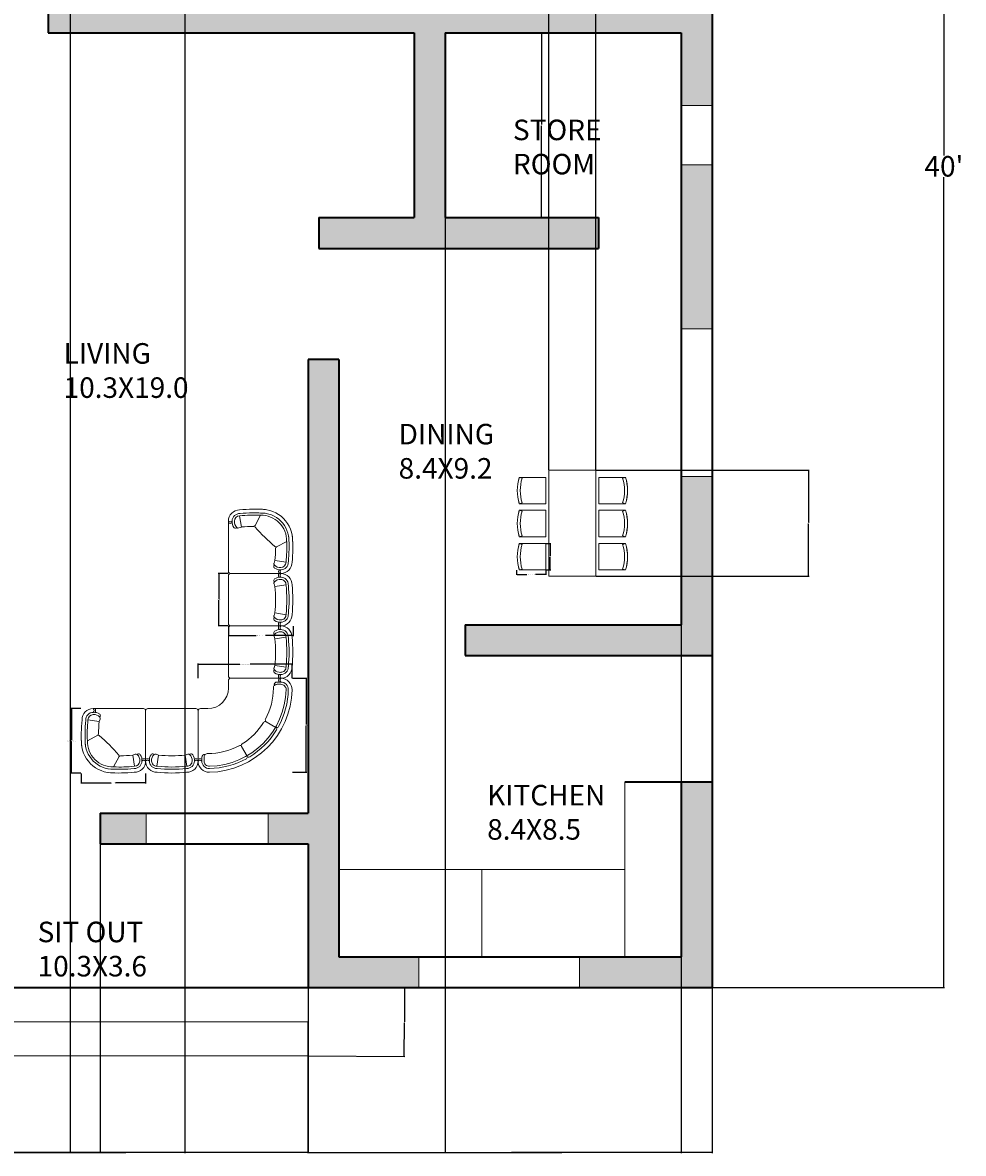
# Model space of a CAD drawing. Units: inches. Extents: x 8 to 486, y -516 to 97.
# Tile 2 of 5: x 211 to 486, y -516 to -185. Entities that reach past the tile are written whole.
import ezdxf

# ---------------------------------------------------------------- set-up
doc = ezdxf.new("R2010")
doc.units = ezdxf.units.IN
doc.header["$MEASUREMENT"] = 0
for name, color, linetype, lineweight in [('A-ANNO-DIMS', 2, 'Continuous', 18), ('A-AREA-IDEN', 7, 'Continuous', 18), ('A-FLOR-CABN', 8, 'Continuous', 18), ('A-FLOR-STRS', 7, 'Continuous', 18), ('A-FURN', 8, 'Continuous', 18), ('A-GLAZ', 4, 'Continuous', 18), ('A-WALL', 7, 'Continuous', 35), ('A-WALL-PATT', 150, 'Continuous', 13)]:
    doc.layers.add(name, color=color, linetype=linetype, lineweight=lineweight)
doc.styles.get("Standard").update_dxf_attribs({"font": 'arial.ttf'})
doc.dimstyles.get("Standard").update_dxf_attribs({"dimtxt": 0.18, "dimasz": 0.18, "dimexe": 0.18, "dimexo": 0.0625, "dimgap": 0.09, "dimtad": 0, "dimtih": 1, "dimtoh": 1, "dimdec": 0, "dimzin": 0, "dimdsep": 46, "dimlunit": 3, "dimtxsty": 'Standard', "dimcen": 0.09, "dimadec": 0, "dimazin": 0, "dimtfac": 1, "dimtdec": 0, "dimtofl": 0, "dimtmove": 0, "dimatfit": 3, "dimfxl": 1, "dimtolj": 1, "dimtzin": 0, "dimarcsym": 0})

# ---------------------------------------------------------------- blocks, each defined once
blk = doc.blocks.new('*D2')
at = {"layer": 'A-ANNO-DIMS', "color": 0, "lineweight": -2, "transparency": 16777216}
for p, q in [((412.19, 12.74), (480.06, 12.74)), ((479.88, 12.56), (479.88, -224.11)), ((479.88, -467.08), (479.88, -230.42)), ((412.19, -467.26), (480.06, -467.26))]:
    blk.add_line(p, q, dxfattribs=at)
at = {"layer": 'A-ANNO-DIMS', "color": 0, "transparency": 16777216}
for points in [[(479.85, 12.56), (479.91, 12.56), (479.88, 12.74)], [(479.85, -467.08), (479.91, -467.08), (479.88, -467.26)]]:
    blk.add_solid(points, dxfattribs=at)
at = {"layer": 'Defpoints', "color": 0, "transparency": 16777216}
for p in [(412.13, 12.74), (412.13, -467.26), (479.88, -467.26)]:
    blk.add_point(p, dxfattribs=at)
at = {"layer": 'A-ANNO-DIMS', "color": 0, "transparency": 16777216, "insert": (479.88, -227.26), "char_height": 6, "attachment_point": 5}
blk.add_mtext("\\A1;40'", dxfattribs=at)
blk = doc.blocks.new('A$C707258B2')
at = {"color": 0}
for p, q in [((0.404, 0.342), (1.074, 0.342)), ((1.104, 0.312), (1.104, 0.212)), ((0.404, 0.292), (0.454, 0.292)), ((0.404, 0.262), (0.454, 0.262)), ((1.479, -0.063), (1.379, -0.063)), ((1.509, -0.763), (1.509, -0.093)), ((0.6, -0.238), (0.47, -0.313)), ((0.929, -0.567), (0.854, -0.697)), ((1.429, -0.763), (1.429, -0.713)), ((1.459, -0.763), (1.459, -0.712))]:
    blk.add_line(p, q, dxfattribs=at)
for centre, radius, start, end in [((0.404, 0.192), 0.15, 90, 181.1754), ((0.378, 0.317), 0.0362, 316.3972, 43.6028), ((0.368, 0.317), 0.0662, 337.8298, 22.1702), ((1.074, 0.312), 0.03, 360, 90), ((1.379, 0.212), 1.125, 181.1754, 268.8246), ((0.404, 0.192), 0.1, 90, 181.1754), ((1.379, 0.212), 1.075, 181.1754, 208.6357), ((0.404, 0.192), 0.07, 90, 181.1754), ((1.379, 0.212), 1.045, 181.1754, 268.8246), ((0.455, 0.256), 0.0357, 345.4262, 90.5555), ((0.454, 0.212), 0.05, 360, 90), ((1.379, 0.212), 0.875, 180, 208.4082), ((1.379, 0.212), 0.275, 180, 270), ((1.479, -0.093), 0.03, 360, 90), ((0.587, -0.216), 0.025, 300, 28.4082), ((0.612, -0.259), 0.025, 31.5918, 120), ((1.379, 0.212), 0.875, 211.5918, 238.4082), ((0.457, -0.291), 0.025, 208.6357, 300), ((0.482, -0.334), 0.025, 120, 211.3643), ((1.379, 0.212), 1.075, 211.3643, 238.6357), ((0.907, -0.555), 0.025, 330, 58.4082), ((0.951, -0.58), 0.025, 61.5918, 150), ((1.379, 0.212), 0.875, 241.5918, 270), ((0.832, -0.685), 0.025, 238.6357, 330), ((0.876, -0.71), 0.025, 150, 241.3643), ((1.379, 0.212), 1.075, 241.3643, 268.8246), ((1.379, -0.713), 0.05, 360, 90), ((1.425, -0.709), 0.0336, 354.6301, 109.3883), ((1.484, -0.799), 0.0662, 67.8298, 112.1702), ((1.484, -0.789), 0.0362, 46.3972, 133.6028), ((1.359, -0.763), 0.15, 268.8246, 360), ((1.359, -0.763), 0.1, 268.8246, 360), ((1.359, -0.763), 0.07, 268.8246, 360)]:
    blk.add_arc(centre, radius, start, end, dxfattribs=at)
blk = doc.blocks.new('part 01')
at = {"color": 0}
for p, q in [((-670, 700), (0, 700)), ((30, 30), (30, 670)), ((-591, 527), (-740, 550)), ((-591, 527), (-579, 561)), ((-591, 173), (-740, 150)), ((-591, 173), (-579, 139)), ((-670, 0), (0, 0))]:
    blk.add_line(p, q, dxfattribs=at)
for centre, radius, start, end in [((-670, 550), 150, 90, 181.1754), ((-670, 550), 100, 90, 181.1754), ((-670, 550), 70, 90, 181.1754), ((-660, 518), 133, 56.0897, 95.6132), ((-696, 675), 36.2, 316.3972, 43.6028), ((-660, 518), 103, 42.0066, 95.6132), ((-706, 675), 66.2, 337.8298, 22.1702), ((-600, 607), 25, 332.9608, 56.0897), ((0, 670), 30, 0, 90), ((1178, 350), 2008, 174.2835, 185.7165), ((1178, 350), 1958, 174.2835, 185.7165), ((1178, 350), 1928, 174.2835, 185.7165), ((1178, 350), 1778, 174.2835, 185.7165), ((-625, 620), 53.2, 321.0017, 332.9608), ((-602, 570), 25, 340, 42.0066), ((-670, 150), 150, 178.8246, 270), ((-670, 150), 100, 178.8246, 270), ((-670, 150), 70, 178.8246, 270), ((-660, 182), 133, 264.3868, 303.9103), ((-660, 182), 103, 264.3868, 317.9934), ((-696, 25), 36.2, 316.3972, 43.6028), ((-706, 25), 66.2, 337.8298, 22.1702), ((-600, 93), 25, 303.9103, 27.0392), ((-602, 130), 25, 317.9934, 20), ((-625, 80), 53.2, 27.0392, 38.9983), ((0, 30), 30, 270, 0)]:
    blk.add_arc(centre, radius, start, end, dxfattribs=at)
blk = doc.blocks.new('part02')
at = {"color": 0}
for p, q in [((0, -670), (0, 0)), ((30, 30), (700, 30)), ((621, -143), (609, -109)), ((621, -143), (770, -120)), ((640, -326), (778, -399)), ((173, -591), (139, -579)), ((173, -591), (150, -740)), ((356, -610), (429, -748))]:
    blk.add_line(p, q, dxfattribs=at)
for centre, radius, start, end in [((30, 0), 30, 90, 180), ((726, 5), 56.2, 153.6122, 206.6666), ((726, 5), 36.2, 136.3972, 223.6028), ((700, -120), 150, 0, 90), ((630, -63), 25, 123.9103, 207.0392), ((655, -50), 53.2, 207.0392, 218.9983), ((632, -100), 25, 137.9934, 200), ((690, -152), 103, 84.3868, 137.9934), ((689, -151), 132, 85.4378, 123.9887), ((-1148, -320), 1778, 0.3836, 5.7165), ((700, -121), 101, 357.5006, 89.858), ((700, -120), 70, 0, 90), ((-1228, -320), 2008, 357.7349, 5.7032), ((-1148, -320), 1958, 355.8657, 5.7165), ((-1148, -320), 2008, 355.818, 5.7165), ((2220, -2190), 2454, 130.6961, 139.3039), ((439, -409), 419, 268.2181, 1.7819), ((439, -409), 369, 268.2181, 1.7819), ((439, -409), 339, 268.2181, 1.7819), ((632, -344), 20, 62, 130.6961), ((650, -308), 20, 180.3836, 242), ((182, -660), 133, 146.0897, 185.6132), ((93, -600), 25, 62.9608, 146.0897), ((182, -660), 103, 132.0066, 185.6132), ((80, -625), 53.2, 51.0017, 62.9608), ((130, -602), 25, 70, 132.0066), ((350, 1178), 1778, 264.2835, 269.6164), ((338, -620), 20, 28, 89.6164), ((374, -602), 20, 139.3039, 208), ((25, -696), 56.2, 63.3334, 116.3878), ((25, -696), 36.2, 46.3972, 133.6028), ((150, -670), 150, 180, 271.1754), ((150, -670), 100, 180, 271.1754), ((150, -670), 70, 180, 270), ((350, 1258), 2008, 264.2968, 272.2651), ((350, 1178), 2008, 264.2835, 274.182), ((350, 1178), 1958, 264.2835, 274.1343)]:
    blk.add_arc(centre, radius, start, end, dxfattribs=at)
blk = doc.blocks.new('CHAIR-DINING')
for p, q in [((0.6, 7.75), (1.42, 7.49)), ((0.6, 0), (1.42, 0.26))]:
    blk.add_line(p, q)
blk.add_lwpolyline([(0.6, 7.75), (8.35, 7.75), (8.35, 0), (0.6, 0, -0.153703), (0.6, 7.75)], format="xyb")
for radius in [12.78, 11.92]:
    blk.add_arc((12.79, 3.88), radius, 162.3544, 197.6456)
blk = doc.blocks.new('*D13')
at = {"layer": 'A-ANNO-DIMS', "color": 0, "lineweight": -2, "transparency": 16777216}
for p, q in [((355.03, -345.29), (355.03, -346.69)), ((355.21, -346.51), (358.03, -346.51)), ((363.4, -346.51), (360.58, -346.51)), ((363.58, -345.29), (363.58, -346.69))]:
    blk.add_line(p, q, dxfattribs=at)
at = {"layer": 'A-ANNO-DIMS', "color": 0, "transparency": 16777216}
for points in [[(355.21, -346.48), (355.21, -346.54), (355.03, -346.51)], [(363.4, -346.48), (363.4, -346.54), (363.58, -346.51)]]:
    blk.add_solid(points, dxfattribs=at)
at = {"layer": 'Defpoints', "color": 0, "transparency": 16777216}
for p in [(355.03, -345.23), (363.58, -345.23), (363.58, -346.51)]:
    blk.add_point(p, dxfattribs=at)
at = {"layer": 'A-ANNO-DIMS', "color": 0, "transparency": 16777216, "insert": (359.3, -346.51), "char_height": 0.18, "attachment_point": 5}
blk.add_mtext('\\A1;CHAIR 0\'-8 1/2" TYP.', dxfattribs=at)
blk = doc.blocks.new('*D14')
at = {"layer": 'A-ANNO-DIMS', "color": 0, "lineweight": -2, "transparency": 16777216}
for p, q in [((363.64, -337.48), (365.04, -337.48)), ((364.86, -337.66), (364.86, -341.17)), ((364.86, -345.05), (364.86, -341.53)), ((363.64, -345.23), (365.04, -345.23))]:
    blk.add_line(p, q, dxfattribs=at)
at = {"layer": 'A-ANNO-DIMS', "color": 0, "transparency": 16777216}
for points in [[(364.83, -337.66), (364.89, -337.66), (364.86, -337.48)], [(364.83, -345.05), (364.89, -345.05), (364.86, -345.23)]]:
    blk.add_solid(points, dxfattribs=at)
at = {"layer": 'Defpoints', "color": 0, "transparency": 16777216}
for p in [(363.58, -337.48), (364.86, -337.48), (363.58, -345.23)]:
    blk.add_point(p, dxfattribs=at)
at = {"layer": 'A-ANNO-DIMS', "color": 0, "transparency": 16777216, "insert": (364.86, -341.35), "char_height": 0.18, "attachment_point": 5}
blk.add_mtext('\\A1;0\'-8" TYP.', dxfattribs=at)
blk = doc.blocks.new('*D15')
at = {"layer": 'A-ANNO-DIMS', "color": 0, "lineweight": -2, "transparency": 16777216}
for p, q in [((270.85, -361.64), (270.85, -364.59)), ((289.73, -361.64), (289.73, -364.59)), ((271.03, -364.41), (278.91, -364.41)), ((289.55, -364.41), (281.67, -364.41))]:
    blk.add_line(p, q, dxfattribs=at)
at = {"layer": 'A-ANNO-DIMS', "color": 0, "transparency": 16777216}
for points in [[(271.03, -364.38), (271.03, -364.44), (270.85, -364.41)], [(289.55, -364.38), (289.55, -364.44), (289.73, -364.41)]]:
    blk.add_solid(points, dxfattribs=at)
at = {"layer": 'Defpoints', "color": 0, "transparency": 16777216}
for p in [(270.85, -361.58), (289.73, -361.58), (270.85, -364.41)]:
    blk.add_point(p, dxfattribs=at)
at = {"layer": 'A-ANNO-DIMS', "color": 0, "transparency": 16777216, "insert": (280.29, -364.41), "char_height": 0.18, "attachment_point": 5}
blk.add_mtext('\\A1;SOFA SEAT 1\'-7" TYP.', dxfattribs=at)
blk = doc.blocks.new('*D16')
at = {"layer": 'A-ANNO-DIMS', "color": 0, "lineweight": -2, "transparency": 16777216}
for p, q in [((270.78, -346.26), (267.83, -346.26)), ((268.01, -346.44), (268.01, -353.74)), ((268.01, -361.4), (268.01, -354.1)), ((270.78, -361.58), (267.83, -361.58))]:
    blk.add_line(p, q, dxfattribs=at)
at = {"layer": 'A-ANNO-DIMS', "color": 0, "transparency": 16777216}
for points in [[(267.98, -346.44), (268.04, -346.44), (268.01, -346.26)], [(267.98, -361.4), (268.04, -361.4), (268.01, -361.58)]]:
    blk.add_solid(points, dxfattribs=at)
at = {"layer": 'Defpoints', "color": 0, "transparency": 16777216}
for p in [(268.01, -346.26), (270.85, -346.26), (270.85, -361.58)]:
    blk.add_point(p, dxfattribs=at)
at = {"layer": 'A-ANNO-DIMS', "color": 0, "transparency": 16777216, "insert": (268.01, -353.92), "char_height": 0.18, "attachment_point": 5}
blk.add_mtext('\\A1;1\'-3 1/2" TYP.', dxfattribs=at)
blk = doc.blocks.new('*D17')
at = {"layer": 'A-ANNO-DIMS', "color": 0, "lineweight": -2, "transparency": 16777216}
for p, q in [((227.73, -385.75), (224.78, -385.75)), ((224.96, -385.93), (224.96, -395.01)), ((224.96, -404.45), (224.96, -395.38)), ((227.73, -404.63), (224.78, -404.63))]:
    blk.add_line(p, q, dxfattribs=at)
at = {"layer": 'A-ANNO-DIMS', "color": 0, "transparency": 16777216}
for points in [[(224.93, -385.93), (224.99, -385.93), (224.96, -385.75)], [(224.93, -404.45), (224.99, -404.45), (224.96, -404.63)]]:
    blk.add_solid(points, dxfattribs=at)
at = {"layer": 'Defpoints', "color": 0, "transparency": 16777216}
for p in [(224.96, -385.75), (227.79, -385.75), (227.79, -404.63)]:
    blk.add_point(p, dxfattribs=at)
at = {"layer": 'A-ANNO-DIMS', "color": 0, "transparency": 16777216, "insert": (224.96, -395.19), "char_height": 0.18, "attachment_point": 5}
blk.add_mtext('\\A1;SOFA END 1\'-7" TYP.', dxfattribs=at)
blk = doc.blocks.new('*D18')
at = {"layer": 'A-ANNO-DIMS', "color": 0, "lineweight": -2, "transparency": 16777216}
for p, q in [((227.79, -404.69), (227.79, -407.64)), ((246.67, -404.69), (246.67, -407.64)), ((227.97, -407.46), (236.6, -407.46)), ((246.49, -407.46), (237.86, -407.46))]:
    blk.add_line(p, q, dxfattribs=at)
at = {"layer": 'A-ANNO-DIMS', "color": 0, "transparency": 16777216}
for points in [[(227.97, -407.43), (227.97, -407.49), (227.79, -407.46)], [(246.49, -407.43), (246.49, -407.49), (246.67, -407.46)]]:
    blk.add_solid(points, dxfattribs=at)
at = {"layer": 'Defpoints', "color": 0, "transparency": 16777216}
for p in [(227.79, -404.63), (246.67, -404.63), (227.79, -407.46)]:
    blk.add_point(p, dxfattribs=at)
at = {"layer": 'A-ANNO-DIMS', "color": 0, "transparency": 16777216, "insert": (237.23, -407.46), "char_height": 0.18, "attachment_point": 5}
blk.add_mtext('\\A1;1\'-7" TYP.', dxfattribs=at)
blk = doc.blocks.new('*D19')
at = {"layer": 'A-ANNO-DIMS', "color": 0, "lineweight": -2, "transparency": 16777216}
for p, q in [((261.99, -376.83), (261.99, -372.59)), ((262.17, -372.77), (274.23, -372.77)), ((289.28, -372.77), (277.22, -372.77)), ((289.46, -376.83), (289.46, -372.59))]:
    blk.add_line(p, q, dxfattribs=at)
at = {"layer": 'A-ANNO-DIMS', "color": 0, "transparency": 16777216}
for points in [[(262.17, -372.74), (262.17, -372.8), (261.99, -372.77)], [(289.28, -372.74), (289.28, -372.8), (289.46, -372.77)]]:
    blk.add_solid(points, dxfattribs=at)
at = {"layer": 'Defpoints', "color": 0, "transparency": 16777216}
for p in [(261.99, -372.77), (261.99, -376.89), (289.46, -376.89)]:
    blk.add_point(p, dxfattribs=at)
at = {"layer": 'A-ANNO-DIMS', "color": 0, "transparency": 16777216, "insert": (275.72, -372.77), "char_height": 0.18, "attachment_point": 5}
blk.add_mtext('\\A1;SOFA CORNER 2\'-3 1/2"', dxfattribs=at)
blk = doc.blocks.new('*D20')
at = {"layer": 'A-ANNO-DIMS', "color": 0, "lineweight": -2, "transparency": 16777216}
for p, q in [((289.52, -376.89), (293.76, -376.89)), ((293.58, -377.07), (293.58, -390.44)), ((293.58, -404.18), (293.58, -390.81)), ((289.52, -404.36), (293.76, -404.36))]:
    blk.add_line(p, q, dxfattribs=at)
at = {"layer": 'A-ANNO-DIMS', "color": 0, "transparency": 16777216}
for points in [[(293.55, -377.07), (293.61, -377.07), (293.58, -376.89)], [(293.55, -404.18), (293.61, -404.18), (293.58, -404.36)]]:
    blk.add_solid(points, dxfattribs=at)
at = {"layer": 'Defpoints', "color": 0, "transparency": 16777216}
for p in [(289.46, -376.89), (293.58, -376.89), (289.46, -404.36)]:
    blk.add_point(p, dxfattribs=at)
at = {"layer": 'A-ANNO-DIMS', "color": 0, "transparency": 16777216, "insert": (293.58, -390.63), "char_height": 0.18, "attachment_point": 5}
blk.add_mtext('\\A1;2\'-3 1/2"', dxfattribs=at)
blk = doc.blocks.new('*D22')
at = {"layer": 'A-ANNO-DIMS', "color": 0, "lineweight": -2, "transparency": 16777216}
for p, q in [((162.13, -487.33), (162.13, -515.64)), ((294.01, -487.33), (294.01, -515.64)), ((162.31, -515.46), (227.68, -515.46)), ((293.83, -515.46), (228.46, -515.46))]:
    blk.add_line(p, q, dxfattribs=at)
at = {"layer": 'A-ANNO-DIMS', "color": 0, "transparency": 16777216}
for points in [[(162.31, -515.43), (162.31, -515.49), (162.13, -515.46)], [(293.83, -515.43), (293.83, -515.49), (294.01, -515.46)]]:
    blk.add_solid(points, dxfattribs=at)
at = {"layer": 'Defpoints', "color": 0, "transparency": 16777216}
for p in [(162.13, -487.26), (294.01, -487.26), (294.01, -515.46)]:
    blk.add_point(p, dxfattribs=at)
at = {"layer": 'A-ANNO-DIMS', "color": 0, "transparency": 16777216, "insert": (228.07, -515.46), "char_height": 0.18, "attachment_point": 5}
blk.add_mtext('\\A1;11\'-0"', dxfattribs=at)
blk = doc.blocks.new('*D23')
at = {"layer": 'A-ANNO-DIMS', "color": 0, "lineweight": -2, "transparency": 16777216}
for p, q in [((294.13, -467.33), (294.13, -515.64)), ((412.13, -467.33), (412.13, -515.64)), ((294.31, -515.46), (352.73, -515.46)), ((411.95, -515.46), (353.53, -515.46))]:
    blk.add_line(p, q, dxfattribs=at)
at = {"layer": 'A-ANNO-DIMS', "color": 0, "transparency": 16777216}
for points in [[(294.31, -515.43), (294.31, -515.49), (294.13, -515.46)], [(411.95, -515.43), (411.95, -515.49), (412.13, -515.46)]]:
    blk.add_solid(points, dxfattribs=at)
at = {"layer": 'Defpoints', "color": 0, "transparency": 16777216}
for p in [(294.13, -467.26), (412.13, -467.26), (412.13, -515.46)]:
    blk.add_point(p, dxfattribs=at)
at = {"layer": 'A-ANNO-DIMS', "color": 0, "transparency": 16777216, "insert": (353.13, -515.46), "char_height": 0.18, "attachment_point": 5}
blk.add_mtext('\\A1;9\'-10"', dxfattribs=at)
blk = doc.blocks.new('*D25')
at = {"layer": 'A-ANNO-DIMS', "color": 0, "lineweight": -2, "transparency": 16777216}
for p, q in [((294.19, -467.27), (322.51, -467.42)), ((322.33, -467.6), (322.27, -477.24)), ((322.21, -487.24), (322.27, -477.61)), ((294.08, -487.27), (322.39, -487.42))]:
    blk.add_line(p, q, dxfattribs=at)
at = {"layer": 'A-ANNO-DIMS', "color": 0, "transparency": 16777216}
for points in [[(322.3, -467.6), (322.36, -467.6), (322.33, -467.42)], [(322.18, -487.24), (322.24, -487.24), (322.21, -487.42)]]:
    blk.add_solid(points, dxfattribs=at)
at = {"layer": 'Defpoints', "color": 0, "transparency": 16777216}
for p in [(294.13, -467.26), (294.01, -487.26), (322.21, -487.42)]:
    blk.add_point(p, dxfattribs=at)
at = {"layer": 'A-ANNO-DIMS', "color": 0, "transparency": 16777216, "insert": (322.27, -477.42), "char_height": 0.18, "attachment_point": 5}
blk.add_mtext('\\A1;1\'-8"', dxfattribs=at)
blk = doc.blocks.new('*D30')
at = {"layer": 'A-ANNO-DIMS', "color": 0, "lineweight": -2, "transparency": 16777216}
for p, q in [((224.63, -103.93), (224.63, -515.64)), ((258.13, -103.93), (258.13, -515.64)), ((224.81, -515.46), (240.84, -515.46)), ((257.95, -515.46), (241.92, -515.46))]:
    blk.add_line(p, q, dxfattribs=at)
at = {"layer": 'A-ANNO-DIMS', "color": 0, "transparency": 16777216}
for points in [[(224.81, -515.43), (224.81, -515.49), (224.63, -515.46)], [(257.95, -515.43), (257.95, -515.49), (258.13, -515.46)]]:
    blk.add_solid(points, dxfattribs=at)
at = {"layer": 'Defpoints', "color": 0, "transparency": 16777216}
for p in [(224.63, -103.87), (258.13, -103.87), (258.13, -515.46)]:
    blk.add_point(p, dxfattribs=at)
at = {"layer": 'A-ANNO-DIMS', "color": 0, "transparency": 16777216, "insert": (241.38, -515.46), "char_height": 0.18, "attachment_point": 5}
blk.add_mtext('\\A1;2\'-9 1/2"', dxfattribs=at)
blk = doc.blocks.new('*D32')
at = {"layer": 'A-ANNO-DIMS', "color": 0, "lineweight": -2, "transparency": 16777216}
for p, q in [((334.13, -188.33), (334.13, -515.64)), ((403.13, -188.33), (403.13, -515.64)), ((334.31, -515.46), (368.3, -515.46)), ((402.95, -515.46), (368.96, -515.46))]:
    blk.add_line(p, q, dxfattribs=at)
at = {"layer": 'A-ANNO-DIMS', "color": 0, "transparency": 16777216}
for points in [[(334.31, -515.43), (334.31, -515.49), (334.13, -515.46)], [(402.95, -515.43), (402.95, -515.49), (403.13, -515.46)]]:
    blk.add_solid(points, dxfattribs=at)
at = {"layer": 'Defpoints', "color": 0, "transparency": 16777216}
for p in [(334.13, -188.26), (403.13, -188.26), (403.13, -515.46)]:
    blk.add_point(p, dxfattribs=at)
at = {"layer": 'A-ANNO-DIMS', "color": 0, "transparency": 16777216, "insert": (368.63, -515.46), "char_height": 0.18, "attachment_point": 5}
blk.add_mtext('\\A1;5\'-9"', dxfattribs=at)
blk = doc.blocks.new('*D33')
at = {"layer": 'A-ANNO-DIMS', "color": 0, "lineweight": -2, "transparency": 16777216}
for p, q in [((334.19, -188.26), (362.51, -188.26)), ((362.33, -188.44), (362.33, -215.08)), ((362.33, -242.08), (362.33, -215.45)), ((334.19, -242.26), (362.51, -242.26))]:
    blk.add_line(p, q, dxfattribs=at)
at = {"layer": 'A-ANNO-DIMS', "color": 0, "transparency": 16777216}
for points in [[(362.3, -188.44), (362.36, -188.44), (362.33, -188.26)], [(362.3, -242.08), (362.36, -242.08), (362.33, -242.26)]]:
    blk.add_solid(points, dxfattribs=at)
at = {"layer": 'Defpoints', "color": 0, "transparency": 16777216}
for p in [(334.13, -188.26), (334.13, -242.26), (362.33, -242.26)]:
    blk.add_point(p, dxfattribs=at)
at = {"layer": 'A-ANNO-DIMS', "color": 0, "transparency": 16777216, "insert": (362.33, -215.26), "char_height": 0.18, "attachment_point": 5}
blk.add_mtext('\\A1;4\'-6"', dxfattribs=at)
blk = doc.blocks.new('*D34')
at = {"layer": 'A-ANNO-DIMS', "color": 0, "lineweight": -2, "transparency": 16777216}
for p, q in [((171.13, -425.33), (171.13, -515.64)), ((233.38, -425.33), (233.38, -515.64)), ((171.31, -515.46), (201.92, -515.46)), ((233.2, -515.46), (202.58, -515.46))]:
    blk.add_line(p, q, dxfattribs=at)
at = {"layer": 'A-ANNO-DIMS', "color": 0, "transparency": 16777216}
for points in [[(171.31, -515.43), (171.31, -515.49), (171.13, -515.46)], [(233.2, -515.43), (233.2, -515.49), (233.38, -515.46)]]:
    blk.add_solid(points, dxfattribs=at)
at = {"layer": 'Defpoints', "color": 0, "transparency": 16777216}
for p in [(171.13, -425.26), (233.38, -425.26), (233.38, -515.46)]:
    blk.add_point(p, dxfattribs=at)
at = {"layer": 'A-ANNO-DIMS', "color": 0, "transparency": 16777216, "insert": (202.25, -515.46), "char_height": 0.18, "attachment_point": 5}
blk.add_mtext('\\A1;5\'-2"', dxfattribs=at)
blk = doc.blocks.new('*D36')
at = {"layer": 'A-ANNO-DIMS', "color": 0, "lineweight": -2, "transparency": 16777216}
for p, q in [((364.45, -315.96), (364.45, 41.12)), ((364.63, 40.94), (371.02, 40.94)), ((378.05, 40.94), (371.66, 40.94)), ((378.23, -315.96), (378.23, 41.12))]:
    blk.add_line(p, q, dxfattribs=at)
at = {"layer": 'A-ANNO-DIMS', "color": 0, "transparency": 16777216}
for points in [[(364.63, 40.97), (364.63, 40.91), (364.45, 40.94)], [(378.05, 40.97), (378.05, 40.91), (378.23, 40.94)]]:
    blk.add_solid(points, dxfattribs=at)
at = {"layer": 'Defpoints', "color": 0, "transparency": 16777216}
for p in [(378.23, 40.94), (364.45, -316.02), (378.23, -316.02)]:
    blk.add_point(p, dxfattribs=at)
at = {"layer": 'A-ANNO-DIMS', "color": 0, "transparency": 16777216, "insert": (371.34, 40.94), "char_height": 0.18, "attachment_point": 5}
blk.add_mtext('\\A1;1\'-2"', dxfattribs=at)
blk = doc.blocks.new('*D37')
at = {"layer": 'A-ANNO-DIMS', "color": 0, "lineweight": -2, "transparency": 16777216}
for p, q in [((378.29, -316.02), (440.51, -316.02)), ((440.33, -316.2), (440.33, -331.34)), ((440.33, -346.84), (440.33, -331.7)), ((378.29, -347.02), (440.51, -347.02))]:
    blk.add_line(p, q, dxfattribs=at)
at = {"layer": 'A-ANNO-DIMS', "color": 0, "transparency": 16777216}
for points in [[(440.3, -316.2), (440.36, -316.2), (440.33, -316.02)], [(440.3, -346.84), (440.36, -346.84), (440.33, -347.02)]]:
    blk.add_solid(points, dxfattribs=at)
at = {"layer": 'Defpoints', "color": 0, "transparency": 16777216}
for p in [(378.23, -316.02), (378.23, -347.02), (440.33, -347.02)]:
    blk.add_point(p, dxfattribs=at)
at = {"layer": 'A-ANNO-DIMS', "color": 0, "transparency": 16777216, "insert": (440.33, -331.52), "char_height": 0.18, "attachment_point": 5}
blk.add_mtext('\\A1;2\'-7"', dxfattribs=at)

msp = doc.modelspace()

# ---------------------------------------------------------------- hatches: boundary and pattern name
at = {"layer": 'A-WALL-PATT'}
h = msp.add_hatch(color=256, dxfattribs=at)
h.dxf.hatch_style = 1
h.paths.add_polyline_path([(91.21, 12.74), (37.13, 12.74), (37.13, -29.65), (46.13, -29.65), (46.13, 3.74), (91.21, 3.74)])
h.paths.add_polyline_path([(211.13, 12.74), (137.85, 12.74), (137.85, 3.74), (182.13, 3.74), (182.13, -73.87), (191.13, -73.87), (191.13, 3.74), (211.13, 3.74)])
h.paths.add_polyline_path([(306.98, 12.74), (234.7, 12.74), (234.7, 3.74), (306.98, 3.74)])
h.paths.add_polyline_path([(267.13, 3.74), (258.13, 3.74), (258.13, -129.26), (267.13, -129.26)])
h.paths.add_polyline_path([(412.13, 12.74), (361.49, 12.74), (361.49, 3.74), (403.13, 3.74), (403.13, -35.28), (412.13, -35.28)])
h.paths.add_polyline_path([(379.01, -120.26), (297.29, -120.26), (297.29, -129.26), (325.13, -129.26), (325.13, -179.26), (218.14, -179.26), (218.14, -188.26), (325.13, -188.26), (325.13, -242.26), (297.29, -242.26), (297.29, -251.26), (379.01, -251.26), (379.01, -242.26), (334.13, -242.26), (334.13, -188.26), (403.13, -188.26), (403.13, -209.46), (412.13, -209.46), (412.13, -162.44), (403.13, -162.44), (403.13, -179.26), (334.13, -179.26), (334.13, -129.26), (379.01, -129.26)])
h.paths.add_polyline_path([(412.13, -70.38), (403.13, -70.38), (403.13, -142.55), (412.13, -142.55)])
h.paths.add_polyline_path([(412.13, -226.8), (403.13, -226.8), (403.13, -274.76), (412.13, -274.76)])
h.paths.add_polyline_path([(412.13, -317.95), (403.13, -317.95), (403.13, -361.26), (339.99, -361.26), (339.99, -370.26), (412.13, -370.26)])
h.paths.add_polyline_path([(412.13, -407.2), (403.13, -407.2), (403.13, -458.26), (373.42, -458.26), (373.42, -467.26), (412.13, -467.26)])
h.paths.add_polyline_path([(326.44, -458.26), (303.13, -458.26), (303.13, -283.74), (294.13, -283.74), (294.13, -416.26), (282.5, -416.26), (282.5, -425.26), (294.13, -425.26), (294.13, -467.26), (326.44, -467.26)])
h.paths.add_polyline_path([(246.84, -416.26), (233.38, -416.26), (233.38, -425.26), (246.84, -425.26)])
h.paths.add_polyline_path([(171.13, -307.26), (171.13, -191.26), (171.13, -182.26), (162.13, -182.26), (162.13, -191.26), (162.13, -307.26), (122.6, -307.26), (122.6, -316.26), (162.13, -316.26), (162.13, -425.26), (171.13, -425.26)])
h.paths.add_polyline_path([(84.39, -307.26), (46.13, -307.26), (46.13, -274.81), (37.13, -274.81), (37.13, -316.26), (84.39, -316.26)])
h.paths.add_polyline_path([(46.13, -191.26), (108.13, -191.26), (108.13, -182.26), (46.13, -182.26), (46.13, -172.25), (37.13, -172.25), (37.13, -224.84), (46.13, -224.84)])
h.paths.add_polyline_path([(191.13, -120.26), (46.13, -120.26), (46.13, -76.77), (37.13, -76.77), (37.13, -150.77), (46.13, -150.77), (46.13, -129.26), (99.13, -129.26), (99.13, -163.77), (108.13, -163.77), (108.13, -129.26), (191.13, -129.26)])

# ---------------------------------------------------------------- linework, layer by layer
at = {"layer": 'A-FLOR-CABN'}
for p, q in [((386.68, -407.2), (386.68, -458.26)), ((386.68, -432.73), (303.13, -432.73)), ((344.9, -432.73), (344.9, -458.26))]:
    msp.add_line(p, q, dxfattribs=at)
at = {"layer": 'A-FLOR-STRS'}
for p, q in [((294.01, -487.26), (294.13, -467.26)), ((162.13, -477.26), (294.07, -477.26)), ((162.13, -487.26), (294.01, -487.26))]:
    msp.add_line(p, q, dxfattribs=at)
at = {"layer": 'A-FURN'}
msp.add_lwpolyline([(378.23, -347.02), (364.45, -347.02), (364.45, -316.02), (378.23, -316.02)], close=True, dxfattribs=at)
at = {"layer": 'A-GLAZ'}
for p, q in [((403.13, -209.46), (412.13, -209.46)), ((403.13, -226.8), (412.13, -226.8)), ((403.13, -274.76), (412.13, -274.76)), ((412.13, -317.95), (403.13, -317.95)), ((246.84, -416.26), (246.84, -425.26)), ((282.5, -416.26), (282.5, -425.26)), ((326.44, -458.26), (326.44, -467.26)), ((373.42, -458.26), (373.42, -467.26))]:
    msp.add_line(p, q, dxfattribs=at)
at = {"layer": 'A-WALL'}
for p, q in [((412.13, 12.74), (412.13, -467.26)), ((218.14, -179.26), (218.14, -188.26)), ((218.14, -188.26), (325.13, -188.26)), ((325.13, -188.26), (325.13, -242.26)), ((334.13, -188.26), (334.13, -242.26)), ((334.13, -188.26), (403.13, -188.26)), ((403.13, -188.26), (403.13, -361.26)), ((297.29, -242.26), (325.13, -242.26)), ((297.29, -242.26), (297.29, -251.26)), ((334.13, -242.26), (379.01, -242.26)), ((379.01, -242.26), (379.01, -251.26)), ((297.29, -251.26), (379.01, -251.26)), ((303.13, -283.74), (294.13, -283.74)), ((294.13, -283.74), (294.13, -416.26)), ((303.13, -283.74), (303.13, -458.26)), ((339.99, -361.26), (403.13, -361.26)), ((339.99, -361.26), (339.99, -370.26)), ((339.99, -370.26), (412.13, -370.26)), ((412.13, -407.2), (386.68, -407.2)), ((403.13, -407.2), (403.13, -458.26)), ((233.38, -416.26), (294.13, -416.26)), ((233.38, -416.26), (233.38, -425.26)), ((233.38, -425.26), (294.13, -425.26)), ((294.13, -425.26), (294.13, -467.26)), ((303.13, -458.26), (403.13, -458.26)), ((37.13, -467.26), (412.13, -467.26))]:
    msp.add_line(p, q, dxfattribs=at)

# ---------------------------------------------------------------- block references
at = {"layer": 'A-FURN'}
for p in [(355.23, -325.91), (355.23, -335.54), (355.23, -345.23)]:
    msp.add_blockref('CHAIR-DINING', p, dxfattribs=at)
at = {"layer": 'A-FURN', "extrusion": (0, 0, -1), "zscale": -1}
for p in [(-387.45, -325.91), (-387.45, -335.54), (-387.45, -345.23)]:
    msp.add_blockref('CHAIR-DINING', p, dxfattribs=at)
at = {"layer": 'A-FURN', "ltscale": 0.03}
for name, p, xscale, yscale, zscale, rotation in [('part02', (271.5, -346.26), 0.0218787882873123, 0.0218787882873123, 0.0218787882873123, 90), ('A$C707258B2', (269.47, -409.91), 21.87878828731224, 21.87878828731224, 21.87878828731224, 90), ('part 01', (246.67, -386.41), -0.0218787882873123, 0.0218787882873123, 0.0218787882873123, 270)]:
    msp.add_blockref(name, p, dxfattribs=dict(at, xscale=xscale, yscale=yscale, zscale=zscale, rotation=rotation))
at = {"layer": 'A-FURN', "ltscale": 0.03, "xscale": -0.0218787882873123, "yscale": 0.0218787882873123, "zscale": 0.0218787882873123}
for name, p in [('part 01', (271.5, -361.58)), ('part 01', (271.5, -376.89)), ('part02', (246.67, -386.41))]:
    msp.add_blockref(name, p, dxfattribs=at)

# ---------------------------------------------------------------- texts
at = {"layer": 'A-AREA-IDEN', "char_height": 6, "attachment_point": 1}
for s, insert in [('STORE\\PROOM', (353.97, -213.62)), ('LIVING\\P10.3X19.0', (222.7, -278.94)), ('DINING\\P8.4X9.2', (320.58, -302.53)), ('KITCHEN\\P8.4X8.5', (346.44, -408.05))]:
    msp.add_mtext(s, dxfattribs=dict(at, insert=insert))
at = {"layer": 'A-AREA-IDEN', "insert": (215.1, -448.02), "char_height": 6, "attachment_point": 1}
msp.add_mtext_dynamic_manual_height_columns('SIT OUT\\P10.3X3.6', width=43.5088, gutter_width=1, heights=[0], dxfattribs=at)

# ---------------------------------------------------------------- dimensions: what is measured, and where the dimension line sits
at = {"layer": 'A-ANNO-DIMS'}
for base, p1, p2, picture, middle in [((378.23, 40.94), (364.45, -316.02), (378.23, -316.02), '*D36', (371.34, 40.94)), ((258.13, -515.46), (224.63, -103.87), (258.13, -103.87), '*D30', (241.38, -515.46)), ((403.13, -515.46), (334.13, -188.26), (403.13, -188.26), '*D32', (368.63, -515.46)), ((233.3763, -515.4649), (171.1266, -425.2649), (233.3763, -425.2649), '*D34', (202.2515, -515.4649)), ((412.13, -515.46), (294.13, -467.26), (412.13, -467.26), '*D23', (353.13, -515.46)), ((294.01, -515.46), (162.13, -487.26), (294.01, -487.26), '*D22', (228.07, -515.46))]:
    dim = msp.add_linear_dim(base=base, p1=p1, p2=p2, dimstyle='Standard', override={"dimdec": 1, "dimlfac": 1, "dimrnd": 0, "dimzin": 1, "dimdsep": 46, "dimlunit": 4, "dimfrac": 2}, dxfattribs=at)
    dim.commit()
    dim.dimension.update_dxf_attribs({"geometry": picture, "text_midpoint": middle})
for base, p1, p2, angle, override, picture, middle in [((479.88, -467.26), (412.13, 12.74), (412.13, -467.26), 90, {"dimtxt": 6, "dimclrd": 0, "dimclre": 0, "dimclrt": 0}, '*D2', (479.88, -227.26)), ((362.33, -242.26), (334.13, -188.26), (334.13, -242.26), 270, {"dimdec": 1, "dimlfac": 1, "dimrnd": 0, "dimzin": 1, "dimdsep": 46, "dimlunit": 4, "dimfrac": 2}, '*D33', (362.33, -215.26)), ((440.33, -347.02), (378.23, -316.02), (378.23, -347.02), 90, {"dimdec": 1, "dimlfac": 1, "dimrnd": 0, "dimzin": 1, "dimdsep": 46, "dimlunit": 4, "dimfrac": 2}, '*D37', (440.33, -331.52)), ((293.58, -376.89), (289.46, -404.36), (289.46, -376.89), 90, {"dimdec": 1, "dimlfac": 1, "dimrnd": 0, "dimzin": 1, "dimdsep": 46, "dimlunit": 4, "dimfrac": 2}, '*D20', (293.58, -390.63)), ((322.21, -487.42), (294.13, -467.26), (294.01, -487.26), 269.6779, {"dimdec": 1, "dimlfac": 1, "dimrnd": 0, "dimzin": 1, "dimdsep": 46, "dimlunit": 4, "dimfrac": 2}, '*D25', (322.27, -477.42))]:
    dim = msp.add_linear_dim(base=base, p1=p1, p2=p2, angle=angle, dimstyle='Standard', override=override, dxfattribs=at)
    dim.commit()
    dim.dimension.update_dxf_attribs({"geometry": picture, "text_midpoint": middle})
for base, p1, p2, angle, text, picture, middle in [((364.8579, -337.4764), (363.5758, -345.2273), (363.5758, -337.4764), 90, '<> TYP.', '*D14', (364.8579, -341.3519)), ((268.01, -346.26), (270.85, -361.58), (270.85, -346.26), 90, '<> TYP.', '*D16', (268.01, -353.92)), ((270.85, -364.41), (289.73, -361.58), (270.85, -361.58), 180, 'SOFA SEAT <> TYP.', '*D15', (280.29, -364.41)), ((261.99, -372.77), (289.46, -376.89), (261.99, -376.89), 180, 'SOFA CORNER <>', '*D19', (275.72, -372.77)), ((224.96, -385.75), (227.79, -404.63), (227.79, -385.75), 90, 'SOFA END <> TYP.', '*D17', (224.96, -395.19)), ((227.79, -407.46), (246.67, -404.63), (227.79, -404.63), 180, '<> TYP.', '*D18', (237.23, -407.46))]:
    dim = msp.add_linear_dim(base=base, p1=p1, p2=p2, angle=angle, text=text, dimstyle='Standard', override={"dimdec": 1, "dimlfac": 1, "dimrnd": 0, "dimzin": 1, "dimdsep": 46, "dimlunit": 4, "dimfrac": 2}, dxfattribs=at)
    dim.commit()
    dim.dimension.update_dxf_attribs({"geometry": picture, "text_midpoint": middle})
dim = msp.add_linear_dim(base=(363.5758, -346.5094), p1=(355.0288, -345.2273), p2=(363.5758, -345.2273), text='CHAIR <> TYP.', dimstyle='Standard', override={"dimdec": 1, "dimlfac": 1, "dimrnd": 0, "dimzin": 1, "dimdsep": 46, "dimlunit": 4, "dimfrac": 2}, dxfattribs=at)
dim.commit()
dim.dimension.update_dxf_attribs({"geometry": '*D13', "text_midpoint": (359.3023, -346.5094)})

doc.saveas('drawing.dxf')
